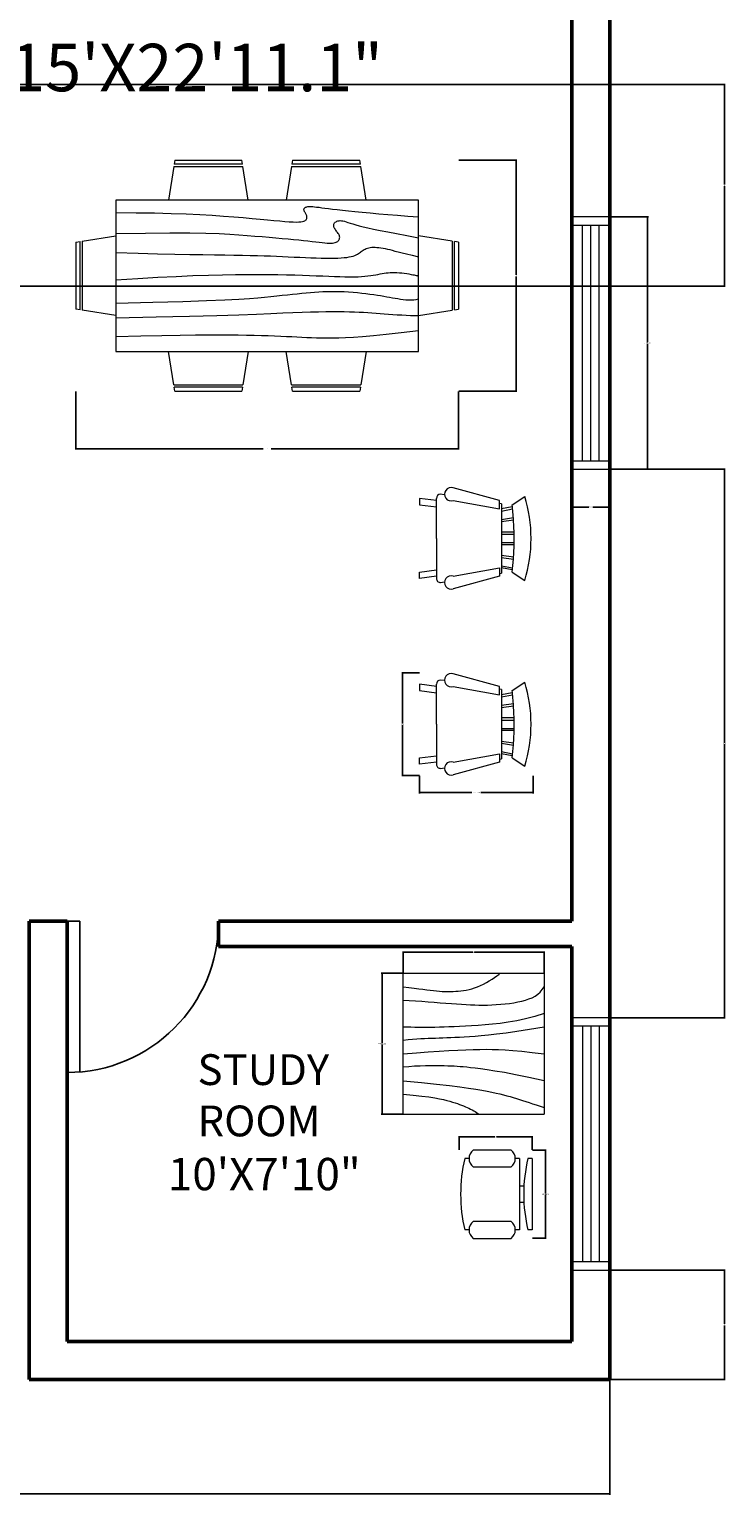
# Model space of a CAD drawing. Units: inches. Extents: x 16 to 443, y 39 to 637.
# Tile 2 of 3: x 278 to 443, y 39 to 387. Entities that reach past the tile are written whole.
import ezdxf

# ---------------------------------------------------------------- set-up
doc = ezdxf.new("R2010")
doc.units = ezdxf.units.IN
for name, color, linetype, lineweight in [('A-ANNO-DIMS', 2, 'Continuous', 18), ('A-AREA-IDEN', 7, 'Continuous', 18), ('A-DOOR', 3, 'Continuous', 25), ('A-FURN', 8, 'Continuous', 18), ('A-GLAZ', 4, 'Continuous', 18), ('A-WALL', 7, 'Continuous', 50)]:
    doc.layers.add(name, color=color, linetype=linetype, lineweight=lineweight)
doc.styles.get("Standard").update_dxf_attribs({"font": 'arial.ttf'})
doc.dimstyles.get("Standard").update_dxf_attribs({"dimtxt": 0.18, "dimasz": 0.18, "dimexe": 0.18, "dimexo": 0.0625, "dimgap": 0.09, "dimtad": 0, "dimtih": 1, "dimtoh": 1, "dimdec": 4, "dimzin": 0, "dimdsep": 46, "dimtxsty": 'Standard', "dimcen": 0.09, "dimadec": 0, "dimazin": 0, "dimtfac": 1, "dimtdec": 4, "dimtofl": 0, "dimtmove": 0, "dimatfit": 3, "dimfxl": 1, "dimtolj": 1, "dimtzin": 0, "dimarcsym": 0})

# ---------------------------------------------------------------- blocks, each defined once
blk = doc.blocks.new('Dining Set - 36 x 72 in.')
for p, q in [((-22.2343, 26.00059), (-23.4847, 17.99762)), ((-22.2304, 26), (-5.7608, 26)), ((-22, 27.5), (-22.1562, 26.50042)), ((-5.8416, 26.5), (-22.1534, 26.5)), ((-22, 27.5), (-6, 27.5)), ((-5.8437, 26.49966), (-6, 27.5)), ((-4.5152, 17.99762), (-5.7655, 25.99926)), ((5.7657, 26.00059), (4.5153, 17.99762)), ((5.7696, 26), (22.2392, 26)), ((6, 27.5), (5.8438, 26.50042)), ((22.1584, 26.5), (5.8466, 26.5)), ((6, 27.5), (22, 27.5)), ((22.1563, 26.49966), (22, 27.5)), ((23.4848, 17.99762), (22.2345, 25.99926)), ((36, 18), (-36, 18)), ((-36, 18), (-36, -18)), ((36, -18), (36, 18)), ((-45.5, 8), (-44.5004, 8.15617)), ((-45.5, 8), (-45.5, -8)), ((-44.5, -8.15843), (-44.5, 8.15338)), ((-44.0006, 8.23428), (-35.9976, 9.48474)), ((-44, 8.23041), (-44, -8.23915)), ((44.0006, 8.23428), (35.9976, 9.48474)), ((44, 8.23041), (44, -8.23915)), ((44.5, -8.15843), (44.5, 8.15338)), ((45.5, 8), (44.5005, 8.15617)), ((45.5, 8), (45.5, -8)), ((-44.4997, -8.15631), (-45.5, -8)), ((-35.9976, -9.48476), (-43.9993, -8.2345)), ((35.9976, -9.48476), (43.9993, -8.2345)), ((44.4997, -8.15631), (45.5, -8)), ((-36, -18), (36, -18)), ((-22.2343, -26.0006), (-23.4847, -17.99762)), ((-4.5152, -17.99762), (-5.7655, -25.99928)), ((5.7657, -26.0006), (4.5153, -17.99762)), ((23.4848, -17.99762), (22.2345, -25.99928)), ((-22.2304, -26), (-5.7608, -26)), ((-22, -27.5), (-22.1562, -26.50044)), ((-5.8416, -26.5), (-22.1534, -26.5)), ((-22, -27.5), (-6, -27.5)), ((-5.8437, -26.49967), (-6, -27.5)), ((5.7696, -26), (22.2392, -26)), ((6, -27.5), (5.8438, -26.50044)), ((22.1584, -26.5), (5.8466, -26.5)), ((6, -27.5), (22, -27.5)), ((22.1563, -26.49967), (22, -27.5))]:
    blk.add_line(p, q)
for points in [[(-36, 15), (-31.1772, 14.97754), (-26.8079, 14.91406), (-22.8538, 14.81543), (-19.276, 14.6875), (-16.0362, 14.53613), (-13.0957, 14.36718), (-10.4159, 14.18652), (-7.9583, 14), (-5.6904, 13.81315), (-3.6035, 13.63021), (-1.6954, 13.45508), (0.0365, 13.29166), (1.5945, 13.14388), (2.9811, 13.01562), (4.1988, 12.9108), (5.25, 12.83333), (6.1393, 12.78613), (6.8802, 12.76823), (7.4883, 12.77767), (7.9792, 12.8125), (8.3685, 12.87077), (8.6719, 12.95052), (8.9049, 13.0498), (9.0833, 13.16666), (9.2205, 13.29899), (9.3216, 13.44401), (9.3895, 13.59879), (9.4271, 13.76041), (9.4373, 13.92594), (9.4232, 14.09245), (9.3875, 14.257), (9.3333, 14.41666), (9.2638, 14.56917), (9.1836, 14.71484), (9.0975, 14.85465), (9.0104, 14.98958), (8.9272, 15.1206), (8.8529, 15.2487), (8.7922, 15.37483), (8.75, 15.5), (8.7305, 15.62467), (8.7344, 15.74739), (8.7617, 15.86621), (8.8125, 15.97916), (8.8867, 16.08431), (8.9844, 16.17968), (9.1055, 16.26334), (9.25, 16.33333), (9.4189, 16.38802), (9.6172, 16.42708), (9.8506, 16.45052), (10.125, 16.45833), (10.4463, 16.45052), (10.8203, 16.42708), (11.2529, 16.38802), (11.75, 16.33333), (12.3184, 16.26318), (12.9694, 16.17838), (13.7151, 16.07991), (14.5677, 15.96875), (15.5395, 15.84586), (16.6426, 15.71224), (17.8893, 15.56884), (19.2917, 15.41666), (20.859, 15.25667), (22.5879, 15.08984), (24.4721, 14.91715), (26.5052, 14.73958), (28.6809, 14.5581), (30.9929, 14.3737), (33.4347, 14.18733), (36, 14)], [(-36, 10), (-28.9766, 10.14274), (-23.1725, 10.20442), (-18.4241, 10.19775), (-14.5677, 10.13541), (-11.4399, 10.03011), (-8.877, 9.89453), (-6.7154, 9.74137), (-4.7917, 9.58333), (-2.9698, 9.43082), (-1.2246, 9.28515), (0.4415, 9.14534), (2.026, 9.01041), (3.5266, 8.87939), (4.9408, 8.7513), (6.266, 8.62516), (7.5, 8.5), (8.6411, 8.37549), (9.6914, 8.2539), (10.6538, 8.13818), (11.5312, 8.03125), (12.3267, 7.93603), (13.043, 7.85547), (13.6831, 7.79248), (14.25, 7.75), (14.7471, 7.7303), (15.1797, 7.73307), (15.5537, 7.75732), (15.875, 7.80208), (16.1494, 7.86637), (16.3828, 7.94922), (16.5811, 8.04964), (16.75, 8.16666), (16.8944, 8.29915), (17.0143, 8.44531), (17.1089, 8.60319), (17.1771, 8.77083), (17.218, 8.94629), (17.2305, 9.1276), (17.2137, 9.31282), (17.1667, 9.5), (17.0895, 9.6875), (16.987, 9.875), (16.8649, 10.0625), (16.7292, 10.25), (16.5856, 10.4375), (16.4401, 10.625), (16.2985, 10.8125), (16.1667, 11), (16.05, 11.18733), (15.9518, 11.3737), (15.8752, 11.5581), (15.8229, 11.73958), (15.798, 11.91715), (15.8034, 12.08984), (15.842, 12.25667), (15.9167, 12.41666), (16.0295, 12.56836), (16.1784, 12.70833), (16.3605, 12.83268), (16.5729, 12.9375), (16.8127, 13.01888), (17.0768, 13.07291), (17.3625, 13.0957), (17.6667, 13.08333), (17.9894, 13.03312), (18.3418, 12.94726), (18.7382, 12.82918), (19.1927, 12.68229), (19.7195, 12.51001), (20.3327, 12.31575), (21.0465, 12.10294), (21.875, 11.875), (22.8357, 11.63354), (23.959, 11.37304), (25.2786, 11.08618), (26.8282, 10.76562), (28.6414, 10.40405), (30.752, 9.99414), (33.1936, 9.52856), (36, 9)], [(-36, 5.5), (-30.7157, 5.3348), (-26.069, 5.20963), (-21.9946, 5.11767), (-18.4271, 5.05208), (-15.3009, 5.00602), (-12.5508, 4.97265), (-10.1112, 4.94515), (-7.9167, 4.91666), (-5.909, 4.88167), (-4.0586, 4.83984), (-2.3429, 4.79215), (-0.7396, 4.73958), (0.7739, 4.6831), (2.22, 4.6237), (3.6213, 4.56233), (5, 4.5), (6.373, 4.43782), (7.7344, 4.3776), (9.0723, 4.32129), (10.375, 4.27083), (11.6309, 4.22819), (12.8281, 4.19531), (13.9551, 4.17415), (15, 4.16666), (15.954, 4.17448), (16.819, 4.19791), (17.6001, 4.23698), (18.3021, 4.29166), (18.9299, 4.36198), (19.4883, 4.44791), (19.9823, 4.54948), (20.4167, 4.66666), (20.7969, 4.79899), (21.1302, 4.94401), (21.4245, 5.09879), (21.6875, 5.26041), (21.9271, 5.42594), (22.1511, 5.59245), (22.3672, 5.757), (22.5834, 5.91666), (22.8065, 6.06868), (23.0404, 6.21093), (23.2879, 6.34147), (23.5521, 6.45833), (23.8358, 6.55957), (24.142, 6.64323), (24.4735, 6.70735), (24.8334, 6.75), (25.2235, 6.76969), (25.642, 6.76692), (26.0858, 6.74267), (26.5521, 6.69791), (27.0379, 6.63362), (27.5404, 6.55078), (28.0565, 6.45036), (28.5834, 6.33333), (29.1242, 6.19987), (29.7071, 6.04687), (30.3661, 5.87044), (31.1354, 5.66666), (32.0493, 5.43164), (33.142, 5.16146), (34.4475, 4.85221), (36, 4.5)], [(-36, -1), (-30.7915, -0.6591), (-26.0195, -0.38216), (-21.6519, -0.16284), (-17.6563, 0.00521), (-14.0005, 0.12833), (-10.6523, 0.21289), (-7.5796, 0.26522), (-4.75, 0.29166), (-2.134, 0.29793), (0.2878, 0.28711), (2.5317, 0.26163), (4.6146, 0.22396), (6.5529, 0.17651), (8.3633, 0.12174), (10.0623, 0.06209), (11.6667, 0), (13.1899, -0.06201), (14.6341, -0.1211), (15.9982, -0.17432), (17.2813, -0.21875), (18.4823, -0.25147), (19.6003, -0.26953), (20.6343, -0.27002), (21.5834, -0.25), (22.4481, -0.20768), (23.2357, -0.14584), (23.9549, -0.06836), (24.6146, 0.02083), (25.2235, 0.11784), (25.7904, 0.21875), (26.3241, 0.31966), (26.8334, 0.41666), (27.3265, 0.50618), (27.8099, 0.58593), (28.2894, 0.65397), (28.7709, 0.70833), (29.2601, 0.74707), (29.763, 0.76823), (30.2855, 0.76985), (30.8334, 0.75), (31.4088, 0.70784), (31.9994, 0.64713), (32.589, 0.57275), (33.1615, 0.48958), (33.7008, 0.4025), (34.1908, 0.3164), (34.6153, 0.23616), (34.9584, 0.16666), (35.2099, 0.11165), (35.3848, 0.07031), (35.504, 0.04069), (35.5886, 0.02083), (35.6594, 0.00879), (35.7377, 0.0026), (35.8442, 0.00032), (36, 0)], [(-36, -6.5), (-27.1843, -6.31267), (-20.084, -6.1263), (-14.469, -5.9419), (-10.1094, -5.76042), (-6.7752, -5.58285), (-4.2363, -5.41016), (-2.2629, -5.24333), (-0.625, -5.08334), (0.8708, -4.93099), (2.2715, -4.78646), (3.5872, -4.64974), (4.8281, -4.52084), (6.0046, -4.39974), (7.127, -4.28646), (8.2053, -4.18099), (9.25, -4.08334), (10.2705, -3.99382), (11.2734, -3.91407), (12.2647, -3.84603), (13.25, -3.79167), (14.2354, -3.75293), (15.2266, -3.73177), (16.2295, -3.73015), (17.25, -3.75), (18.2912, -3.79248), (19.3451, -3.85547), (20.4009, -3.93604), (21.4479, -4.03125), (22.4754, -4.13819), (23.4727, -4.25391), (24.4289, -4.37549), (25.3334, -4.5), (26.1785, -4.62492), (26.9694, -4.74935), (27.7145, -4.87281), (28.4219, -4.99479), (29.1, -5.11483), (29.7572, -5.23242), (30.4016, -5.34709), (31.0417, -5.45834), (31.6837, -5.56437), (32.3262, -5.65821), (32.9658, -5.73153), (33.599, -5.77604), (34.2224, -5.78345), (34.8327, -5.74545), (35.4264, -5.65373), (36, -5.5)], [(-36, -10), (-26.4022, -9.81299), (-18.4675, -9.62891), (-11.9839, -9.45069), (-6.7396, -9.28125), (-2.5226, -9.12354), (0.8789, -8.98047), (3.6769, -8.85498), (6.0833, -8.75), (8.2767, -8.66765), (10.3021, -8.60677), (12.1712, -8.56543), (13.8958, -8.54167), (15.4876, -8.53353), (16.9583, -8.53907), (18.3197, -8.55632), (19.5834, -8.58334), (20.7616, -8.61841), (21.8685, -8.66081), (22.9188, -8.71004), (23.9271, -8.76563), (24.9081, -8.82707), (25.8763, -8.89388), (26.8465, -8.96558), (27.8334, -9.04167), (28.8474, -9.12118), (29.8828, -9.20117), (30.93, -9.27824), (31.9792, -9.34896), (33.0205, -9.40991), (34.0443, -9.45768), (35.0407, -9.48885), (36, -9.5)], [(-36, -14.5), (-30.0881, -14.33513), (-25.0332, -14.21224), (-20.7312, -14.12647), (-17.0781, -14.07292), (-13.97, -14.04671), (-11.3027, -14.04297), (-8.9724, -14.05681), (-6.875, -14.08334), (-4.9224, -14.11833), (-3.0905, -14.16016), (-1.3709, -14.20785), (0.2448, -14.26042), (1.7647, -14.3169), (3.1973, -14.3763), (4.5507, -14.43767), (5.8333, -14.5), (7.0554, -14.5621), (8.235, -14.62175), (9.3922, -14.67652), (10.5469, -14.72396), (11.7192, -14.76164), (12.929, -14.78711), (14.1965, -14.79794), (15.5417, -14.79167), (16.9933, -14.76424), (18.6152, -14.70508), (20.4804, -14.60197), (22.6615, -14.44271), (25.2312, -14.21509), (28.2624, -13.9069), (31.8277, -13.50594), (36, -13)]]:
    blk.add_lwpolyline(points)
blk = doc.blocks.new('Chair - Rocking')
for p, q in [((-8, -4.5), (-10, -1.5)), ((8, -4.5), (10, -1.5)), ((-7.5, -4.5), (-7, -7)), ((-6.5, -7), (-7.02225, -4.43)), ((-4.5, -7), (-4.96674, -4.19951)), ((-4, -7), (-4.40532, -4.16272)), ((-1.5, -4.05012), (-1.5, -7)), ((-1, -7), (-1, -4.05012)), ((1, -7), (1, -4.04655)), ((1.5, -4.05012), (1.5, -7)), ((4, -7), (4.40187, -4.18694)), ((4.5, -7), (4.96761, -4.19437)), ((6.5, -7), (7, -4.4057)), ((7.5, -4.5), (7, -7)), ((-9, -7.5), (-12, -18.49999)), ((-7, -7.5), (-9, -7.5)), ((-9, -18.49999), (-7, -7.5)), ((-8.23428, -6.99939), (-8.3093, -7.47958)), ((-8.23041, -7), (8.23915, -7)), ((7, -7.5), (9, -7.5)), ((9, -18.49999), (7, -7.5)), ((8.31071, -7.48854), (8.23449, -7.00073)), ((9, -7.5), (12, -18.49999)), ((-10.36644, -20.64523), (-10.5, -21.49999)), ((10.5, -21.49999), (10.3575, -20.58798)), ((-9, -22.49999), (-9.5, -26.49999)), ((0, -22.49999), (-9.5, -22.49999)), ((-8, -26.49999), (-7.5, -22.49999)), ((0, -22.49999), (9.5, -22.49999)), ((8, -26.49999), (7.5, -22.49999)), ((9, -22.49999), (9.5, -26.49999)), ((-9.5, -26.49999), (-8, -26.49999)), ((9.5, -26.49999), (8, -26.49999))]:
    blk.add_line(p, q)
for centre, radius, start, end in [((0, -34.08333), 34.08333, 72.93847, 107.0615), ((0, -68.25004), 64.25, 93.92211, 97.15267), ((0, -68.25004), 64.25, 82.84733, 93.92211), ((-10.5, -18.99999), 1.58114, 161.5651, 18.43495), ((10.5, -18.99999), 1.58114, 161.5651, 18.43495), ((-9.5, -21.49999), 1, 180, 270), ((9.5, -21.49999), 1, 270, 0)]:
    blk.add_arc(centre, radius, start, end)
blk = doc.blocks.new('Chair - Desk')
for p, q in [((-8.5, 0), (-8.5, -1)), ((-8.5, 0), (8.5, 0)), ((8.5, 0), (8.5, -1)), ((-8.5, -3), (-8.5, -4)), ((-8.5, -3), (8.5, -3)), ((-2, -3), (-2, -1.9355)), ((2, -1.9576), (2, -3)), ((8.5, -3), (8.5, -4)), ((-10.5, -5), (-10.5, -14)), ((-6.5, -14), (-6.5, -5)), ((6.5, -5), (6.5, -14)), ((10.5, -14), (10.5, -5)), ((-8.5, -15), (-8.5, -16)), ((8.5, -15), (8.5, -16))]:
    blk.add_line(p, q)
for centre, radius, start, end in [((0, 34.625), 36.625, 256.5803, 283.4197), ((-8.5, -6.5), 2.5, 36.8699, 143.1301), ((8.5, -6.5), 2.5, 36.8699, 143.1301), ((-8.5, -12.5), 2.5, 216.8699, 323.1301), ((0, 19.625), 36.625, 256.5803, 283.4197), ((8.5, -12.5), 2.5, 216.8699, 323.1301)]:
    blk.add_arc(centre, radius, start, end)
blk = doc.blocks.new('Table - Square Woodgrain 42 x 42 in.')
blk.add_line((0, -42), (42, -42))
for points in [[(0, -4), (1.704, -4.2172), (3.2358, -4.4188), (4.615, -4.604), (5.8615, -4.7721), (6.9951, -4.9224), (8.0357, -5.0541), (9.0031, -5.1667), (9.9171, -5.2594), (10.7951, -5.3316), (11.6445, -5.3836), (12.4702, -5.4157), (13.277, -5.4283), (14.0698, -5.4217), (14.8535, -5.3964), (15.6331, -5.3526), (16.4133, -5.2908), (17.1986, -5.2103), (17.9913, -5.1062), (18.793, -4.9727), (19.6056, -4.8038), (20.4307, -4.5937), (21.2701, -4.3365), (22.1256, -4.0262), (22.9989, -3.6571), (23.888, -3.2272), (24.7756, -2.7516), (25.6408, -2.2491), (26.4624, -1.7387), (27.2195, -1.2395), (27.891, -0.7703), (28.456, -0.3501), (28.8934, 0.002)], [(0, -42), (0, 0), (42, 0), (42, -42)], [(0, -8), (1.8203, -8.1001), (3.6741, -8.2149), (5.5411, -8.3408), (7.4011, -8.4741), (9.2339, -8.6112), (11.0193, -8.7484), (12.7371, -8.8821), (14.3671, -9.0086), (15.8954, -9.1246), (17.3337, -9.2278), (18.6997, -9.3159), (20.0116, -9.387), (21.2871, -9.4389), (22.5442, -9.4696), (23.8008, -9.477), (25.0749, -9.459), (26.3791, -9.4137), (27.7049, -9.3403), (29.0383, -9.2382), (30.3655, -9.1068), (31.6728, -8.9455), (32.9461, -8.7535), (34.1717, -8.5304), (35.3358, -8.2756), (36.4268, -7.9863), (37.443, -7.6521), (38.3849, -7.2603), (39.253, -6.7986), (40.048, -6.2542), (40.7705, -5.6147), (41.421, -4.8674), (42, -4)], [(42, -12), (39.1784, -12.8621), (36.4519, -13.5654), (33.8246, -14.1294), (31.3004, -14.5731), (28.8832, -14.9161), (26.577, -15.1775), (24.3858, -15.3768), (22.3136, -15.5332), (20.3622, -15.6632), (18.5254, -15.7718), (16.7947, -15.8612), (15.1618, -15.9338), (13.6183, -15.9916), (12.1558, -16.0369), (10.7659, -16.0718), (9.4403, -16.0987), (8.1703, -16.1191), (6.9461, -16.1325), (5.7577, -16.1377), (4.595, -16.1335), (3.4479, -16.1188), (2.3064, -16.0924), (1.1604, -16.0532), (0, -16)], [(42, -16), (37.6529, -16.7365), (33.8802, -17.329), (30.6179, -17.7961), (27.8015, -18.1561), (25.3668, -18.4275), (23.2497, -18.6288), (21.3859, -18.7785), (19.7111, -18.8949), (18.1693, -18.9939), (16.7375, -19.0795), (15.401, -19.1534), (14.1449, -19.217), (12.9544, -19.2717), (11.8148, -19.3191), (10.7113, -19.3606), (9.6291, -19.3976), (8.5534, -19.4323), (7.47, -19.4689), (6.3643, -19.5122), (5.222, -19.5672), (4.0288, -19.6386), (2.7703, -19.7313), (1.4321, -19.8501), (0, -20)], [(0, -24), (3.9243, -23.6805), (7.4766, -23.4138), (10.6891, -23.1954), (13.5943, -23.0205), (16.2247, -22.8847), (18.6125, -22.7832), (20.7903, -22.7116), (22.7903, -22.6651), (24.6563, -22.642), (26.4764, -22.6507), (28.35, -22.7024), (30.3766, -22.8084), (32.6555, -22.98), (35.2861, -23.2283), (38.3678, -23.5645), (42, -24)], [(42, -32), (37.392, -31.017), (33.4585, -30.2231), (30.1291, -29.5949), (27.3334, -29.109), (25.0009, -28.742), (23.0612, -28.4707), (21.4439, -28.2716), (20.0786, -28.1215), (18.8998, -28.0002), (17.8609, -27.9014), (16.9206, -27.8219), (16.0371, -27.7588), (15.1691, -27.709), (14.2748, -27.6693), (13.3128, -27.6368), (12.2415, -27.6083), (11.0295, -27.5824), (9.6867, -27.5643), (8.233, -27.5608), (6.6884, -27.5787), (5.0728, -27.6248), (3.4062, -27.7058), (1.7086, -27.8286), (0, -28)], [(0, -32), (5.4026, -32.5358), (9.9494, -33.019), (13.7424, -33.4553), (16.8834, -33.8505), (19.4743, -34.2106), (21.6171, -34.5413), (23.4136, -34.8486), (24.9657, -35.1382), (26.3614, -35.4156), (27.6332, -35.6841), (28.7995, -35.9467), (29.8788, -36.2064), (30.8897, -36.4661), (31.8507, -36.7288), (32.7802, -36.9973), (33.6968, -37.2747), (34.6175, -37.5635), (35.5531, -37.8651), (36.5128, -38.1805), (37.506, -38.5108), (38.5421, -38.8568), (39.6302, -39.2197), (40.7797, -39.6004), (42, -40)], [(0, -36), (3.0098, -36.2857), (5.5354, -36.5643), (7.6368, -36.8359), (9.374, -37.1009), (10.807, -37.3597), (11.9957, -37.6126), (13.0002, -37.8599), (13.8804, -38.102), (14.6874, -38.3393), (15.4365, -38.5729), (16.1338, -38.8041), (16.7858, -39.0341), (17.3987, -39.264), (17.9787, -39.4952), (18.5322, -39.7288), (19.0655, -39.9662), (19.5832, -40.2081), (20.0842, -40.4544), (20.5657, -40.7046), (21.0249, -40.9581), (21.459, -41.2144), (21.8653, -41.4731), (22.2409, -41.7335), (22.5831, -41.9951)]]:
    blk.add_lwpolyline(points)
blk = doc.blocks.new('WIN-60IN')
for p, q in [((0, 60), (0, 0)), ((9, 60), (0, 60)), ((9, 0), (9, 60)), ((9, 58), (0, 58)), ((2.5, 58), (2.5, 2)), ((4.5, 58), (4.5, 2)), ((6.5, 58), (6.5, 2)), ((0, 2), (9, 2)), ((0, 0), (9, 0))]:
    blk.add_line(p, q)
blk = doc.blocks.new('DOOR-SINGLE-36IN')
for p, q in [((33, 36), (33, 0)), ((36, 36), (36, 0)), ((36, 0), (33, 0))]:
    blk.add_line(p, q)
blk.add_arc((36, 0), 36, 90, 180)
blk = doc.blocks.new('*D15')
at = {"layer": 'A-ANNO-DIMS', "color": 0, "lineweight": -2, "transparency": 16777216}
for p, q in [((415.81, 342.58), (424.93, 342.58)), ((424.75, 342.4), (424.75, 312.76)), ((424.75, 282.76), (424.75, 312.4)), ((415.81, 282.58), (424.93, 282.58))]:
    blk.add_line(p, q, dxfattribs=at)
at = {"layer": 'A-ANNO-DIMS', "color": 0, "transparency": 16777216}
for points in [[(424.72, 342.4), (424.78, 342.4), (424.75, 342.58)], [(424.72, 282.76), (424.78, 282.76), (424.75, 282.58)]]:
    blk.add_solid(points, dxfattribs=at)
at = {"layer": 'Defpoints', "color": 0, "transparency": 16777216}
for p in [(415.75, 342.58), (415.75, 282.58), (424.75, 282.58)]:
    blk.add_point(p, dxfattribs=at)
at = {"layer": 'A-ANNO-DIMS', "color": 0, "transparency": 16777216, "insert": (424.75, 312.58), "char_height": 0.18, "attachment_point": 5}
blk.add_mtext('\\A1;WINDOW 60 TYP.', dxfattribs=at)
blk = doc.blocks.new('*D16')
at = {"layer": 'A-ANNO-DIMS', "color": 0, "lineweight": -2, "transparency": 16777216}
for p, q in [((406.75, 282.52), (406.75, 273.4)), ((415.75, 282.52), (415.75, 273.4)), ((406.93, 273.58), (410.79, 273.58)), ((415.57, 273.58), (411.71, 273.58))]:
    blk.add_line(p, q, dxfattribs=at)
at = {"layer": 'A-ANNO-DIMS', "color": 0, "transparency": 16777216}
for points in [[(406.93, 273.61), (406.93, 273.55), (406.75, 273.58)], [(415.57, 273.61), (415.57, 273.55), (415.75, 273.58)]]:
    blk.add_solid(points, dxfattribs=at)
at = {"layer": 'Defpoints', "color": 0, "transparency": 16777216}
for p in [(406.75, 282.58), (415.75, 282.58), (406.75, 273.58)]:
    blk.add_point(p, dxfattribs=at)
at = {"layer": 'A-ANNO-DIMS', "color": 0, "transparency": 16777216, "insert": (411.25, 273.58), "char_height": 0.18, "attachment_point": 5}
blk.add_mtext('\\A1;9 TYP.', dxfattribs=at)
blk = doc.blocks.new('*D29')
at = {"layer": 'A-ANNO-DIMS', "color": 0, "lineweight": -2, "transparency": 16777216}
for p, q in [((370.54, 209.63), (370.54, 205.47)), ((397.54, 209.63), (397.54, 205.47)), ((370.72, 205.65), (382.94, 205.65)), ((397.36, 205.65), (385.13, 205.65))]:
    blk.add_line(p, q, dxfattribs=at)
at = {"layer": 'A-ANNO-DIMS', "color": 0, "transparency": 16777216}
for points in [[(370.72, 205.68), (370.72, 205.62), (370.54, 205.65)], [(397.36, 205.68), (397.36, 205.62), (397.54, 205.65)]]:
    blk.add_solid(points, dxfattribs=at)
at = {"layer": 'Defpoints', "color": 0, "transparency": 16777216}
for p in [(370.54, 209.7), (397.54, 209.7), (397.54, 205.65)]:
    blk.add_point(p, dxfattribs=at)
at = {"layer": 'A-ANNO-DIMS', "color": 0, "transparency": 16777216, "insert": (384.04, 205.65), "char_height": 0.18, "attachment_point": 5}
blk.add_mtext('\\A1;ROCKER 27 TYP.', dxfattribs=at)
blk = doc.blocks.new('*D30')
at = {"layer": 'A-ANNO-DIMS', "color": 0, "lineweight": -2, "transparency": 16777216}
for p, q in [((370.48, 234.13), (366.31, 234.13)), ((366.49, 233.95), (366.49, 222.09)), ((366.49, 209.88), (366.49, 221.73)), ((370.48, 209.7), (366.31, 209.7))]:
    blk.add_line(p, q, dxfattribs=at)
at = {"layer": 'A-ANNO-DIMS', "color": 0, "transparency": 16777216}
for points in [[(366.46, 233.95), (366.52, 233.95), (366.49, 234.13)], [(366.46, 209.88), (366.52, 209.88), (366.49, 209.7)]]:
    blk.add_solid(points, dxfattribs=at)
at = {"layer": 'Defpoints', "color": 0, "transparency": 16777216}
for p in [(370.54, 234.13), (366.49, 209.7), (370.54, 209.7)]:
    blk.add_point(p, dxfattribs=at)
at = {"layer": 'A-ANNO-DIMS', "color": 0, "transparency": 16777216, "insert": (366.49, 221.91), "char_height": 0.18, "attachment_point": 5}
blk.add_mtext('\\A1;24 TYP.', dxfattribs=at)
blk = doc.blocks.new('*D33')
at = {"layer": 'A-ANNO-DIMS', "color": 0, "lineweight": -2, "transparency": 16777216}
for p, q in [((288.81, 301.05), (288.81, 287.28)), ((379.81, 301.05), (379.81, 287.28)), ((288.99, 287.46), (333.36, 287.46)), ((379.63, 287.46), (335.26, 287.46))]:
    blk.add_line(p, q, dxfattribs=at)
at = {"layer": 'A-ANNO-DIMS', "color": 0, "transparency": 16777216}
for points in [[(288.99, 287.49), (288.99, 287.43), (288.81, 287.46)], [(379.63, 287.49), (379.63, 287.43), (379.81, 287.46)]]:
    blk.add_solid(points, dxfattribs=at)
at = {"layer": 'Defpoints', "color": 0, "transparency": 16777216}
for p in [(288.81, 301.11), (379.81, 301.11), (379.81, 287.46)]:
    blk.add_point(p, dxfattribs=at)
at = {"layer": 'A-ANNO-DIMS', "color": 0, "transparency": 16777216, "insert": (334.31, 287.46), "char_height": 0.18, "attachment_point": 5}
blk.add_mtext('\\A1;DINING SET 91', dxfattribs=at)
blk = doc.blocks.new('*D34')
at = {"layer": 'A-ANNO-DIMS', "color": 0, "lineweight": -2, "transparency": 16777216}
for p, q in [((379.87, 356.11), (393.64, 356.11)), ((393.46, 355.93), (393.46, 328.79)), ((393.46, 301.29), (393.46, 328.43)), ((379.87, 301.11), (393.64, 301.11))]:
    blk.add_line(p, q, dxfattribs=at)
at = {"layer": 'A-ANNO-DIMS', "color": 0, "transparency": 16777216}
for points in [[(393.43, 355.93), (393.49, 355.93), (393.46, 356.11)], [(393.43, 301.29), (393.49, 301.29), (393.46, 301.11)]]:
    blk.add_solid(points, dxfattribs=at)
at = {"layer": 'Defpoints', "color": 0, "transparency": 16777216}
for p in [(379.81, 356.11), (393.46, 356.11), (379.81, 301.11)]:
    blk.add_point(p, dxfattribs=at)
at = {"layer": 'A-ANNO-DIMS', "color": 0, "transparency": 16777216, "insert": (393.46, 328.61), "char_height": 0.18, "attachment_point": 5}
blk.add_mtext('\\A1;55', dxfattribs=at)
blk = doc.blocks.new('*D41')
at = {"layer": 'A-ANNO-DIMS', "color": 0, "lineweight": -2, "transparency": 16777216}
for p, q in [((397.35, 120.63), (400.62, 120.63)), ((400.44, 120.45), (400.44, 110.31)), ((400.44, 99.81), (400.44, 109.94)), ((397.35, 99.63), (400.62, 99.63))]:
    blk.add_line(p, q, dxfattribs=at)
at = {"layer": 'A-ANNO-DIMS', "color": 0, "transparency": 16777216}
for points in [[(400.41, 120.45), (400.47, 120.45), (400.44, 120.63)], [(400.41, 99.81), (400.47, 99.81), (400.44, 99.63)]]:
    blk.add_solid(points, dxfattribs=at)
at = {"layer": 'Defpoints', "color": 0, "transparency": 16777216}
for p in [(397.29, 120.63), (397.29, 99.63), (400.44, 99.63)]:
    blk.add_point(p, dxfattribs=at)
at = {"layer": 'A-ANNO-DIMS', "color": 0, "transparency": 16777216, "insert": (400.44, 110.13), "char_height": 0.18, "attachment_point": 5}
blk.add_mtext('\\A1;DESK CHAIR 21', dxfattribs=at)
blk = doc.blocks.new('*D42')
at = {"layer": 'A-ANNO-DIMS', "color": 0, "lineweight": -2, "transparency": 16777216}
for p, q in [((379.95, 120.69), (379.95, 123.96)), ((380.13, 123.78), (388.41, 123.78)), ((397.11, 123.78), (388.83, 123.78)), ((397.29, 120.69), (397.29, 123.96))]:
    blk.add_line(p, q, dxfattribs=at)
at = {"layer": 'A-ANNO-DIMS', "color": 0, "transparency": 16777216}
for points in [[(380.13, 123.81), (380.13, 123.75), (379.95, 123.78)], [(397.11, 123.81), (397.11, 123.75), (397.29, 123.78)]]:
    blk.add_solid(points, dxfattribs=at)
at = {"layer": 'Defpoints', "color": 0, "transparency": 16777216}
for p in [(397.29, 123.78), (379.95, 120.63), (397.29, 120.63)]:
    blk.add_point(p, dxfattribs=at)
at = {"layer": 'A-ANNO-DIMS', "color": 0, "transparency": 16777216, "insert": (388.62, 123.78), "char_height": 0.18, "attachment_point": 5}
blk.add_mtext('\\A1;17', dxfattribs=at)
blk = doc.blocks.new('*D43')
at = {"layer": 'A-ANNO-DIMS', "color": 0, "lineweight": -2, "transparency": 16777216}
for p, q in [((366.58, 162.67), (361.43, 162.67)), ((361.61, 162.49), (361.61, 146.09)), ((361.61, 129.31), (361.61, 145.72)), ((366.58, 129.13), (361.43, 129.13))]:
    blk.add_line(p, q, dxfattribs=at)
at = {"layer": 'A-ANNO-DIMS', "color": 0, "transparency": 16777216}
for points in [[(361.58, 162.49), (361.64, 162.49), (361.61, 162.67)], [(361.58, 129.31), (361.64, 129.31), (361.61, 129.13)]]:
    blk.add_solid(points, dxfattribs=at)
at = {"layer": 'Defpoints', "color": 0, "transparency": 16777216}
for p in [(361.61, 162.67), (366.64, 162.67), (366.64, 129.13)]:
    blk.add_point(p, dxfattribs=at)
at = {"layer": 'A-ANNO-DIMS', "color": 0, "transparency": 16777216, "insert": (361.61, 145.9), "char_height": 0.18, "attachment_point": 5}
blk.add_mtext('\\A1;STUDY TABLE 34', dxfattribs=at)
blk = doc.blocks.new('*D44')
at = {"layer": 'A-ANNO-DIMS', "color": 0, "lineweight": -2, "transparency": 16777216}
for p, q in [((366.64, 162.73), (366.64, 167.88)), ((366.82, 167.7), (383.19, 167.7)), ((399.99, 167.7), (383.62, 167.7)), ((400.17, 162.73), (400.17, 167.88))]:
    blk.add_line(p, q, dxfattribs=at)
at = {"layer": 'A-ANNO-DIMS', "color": 0, "transparency": 16777216}
for points in [[(366.82, 167.73), (366.82, 167.67), (366.64, 167.7)], [(399.99, 167.73), (399.99, 167.67), (400.17, 167.7)]]:
    blk.add_solid(points, dxfattribs=at)
at = {"layer": 'Defpoints', "color": 0, "transparency": 16777216}
for p in [(400.17, 167.7), (366.64, 162.67), (400.17, 162.67)]:
    blk.add_point(p, dxfattribs=at)
at = {"layer": 'A-ANNO-DIMS', "color": 0, "transparency": 16777216, "insert": (383.41, 167.7), "char_height": 0.18, "attachment_point": 5}
blk.add_mtext('\\A1;34', dxfattribs=at)
blk = doc.blocks.new('*D45')
at = {"layer": 'A-ANNO-DIMS', "color": 0, "lineweight": -2, "transparency": 16777216}
for p, q in [((43.75, 165.02), (43.75, 38.65)), ((415.75, 66.02), (415.75, 38.65)), ((43.93, 38.83), (229.46, 38.83)), ((415.57, 38.83), (230.04, 38.83))]:
    blk.add_line(p, q, dxfattribs=at)
at = {"layer": 'A-ANNO-DIMS', "color": 0, "transparency": 16777216}
for points in [[(43.93, 38.86), (43.93, 38.8), (43.75, 38.83)], [(415.57, 38.86), (415.57, 38.8), (415.75, 38.83)]]:
    blk.add_solid(points, dxfattribs=at)
at = {"layer": 'Defpoints', "color": 0, "transparency": 16777216}
for p in [(43.75, 165.08), (415.75, 66.08), (415.75, 38.83)]:
    blk.add_point(p, dxfattribs=at)
at = {"layer": 'A-ANNO-DIMS', "color": 0, "transparency": 16777216, "insert": (229.75, 38.83), "char_height": 0.18, "attachment_point": 5}
blk.add_mtext('\\A1;372', dxfattribs=at)
blk = doc.blocks.new('*D56')
at = {"layer": 'A-ANNO-DIMS', "color": 0, "lineweight": -2, "transparency": 16777216}
for p, q in [((415.81, 92.08), (443.18, 92.08)), ((443, 91.9), (443, 79.26)), ((443, 66.26), (443, 78.9)), ((415.81, 66.08), (443.18, 66.08))]:
    blk.add_line(p, q, dxfattribs=at)
at = {"layer": 'A-ANNO-DIMS', "color": 0, "transparency": 16777216}
for points in [[(442.97, 91.9), (443.03, 91.9), (443, 92.08)], [(442.97, 66.26), (443.03, 66.26), (443, 66.08)]]:
    blk.add_solid(points, dxfattribs=at)
at = {"layer": 'Defpoints', "color": 0, "transparency": 16777216}
for p in [(415.75, 92.08), (443, 92.08), (415.75, 66.08)]:
    blk.add_point(p, dxfattribs=at)
at = {"layer": 'A-ANNO-DIMS', "color": 0, "transparency": 16777216, "insert": (443, 79.08), "char_height": 0.18, "attachment_point": 5}
blk.add_mtext('\\A1;26', dxfattribs=at)
blk = doc.blocks.new('*D57')
at = {"layer": 'A-ANNO-DIMS', "color": 0, "lineweight": -2, "transparency": 16777216}
for p, q in [((415.81, 282.58), (443.18, 282.58)), ((443, 282.4), (443, 217.51)), ((443, 152.26), (443, 217.15)), ((415.81, 152.08), (443.18, 152.08))]:
    blk.add_line(p, q, dxfattribs=at)
at = {"layer": 'A-ANNO-DIMS', "color": 0, "transparency": 16777216}
for points in [[(442.97, 282.4), (443.03, 282.4), (443, 282.58)], [(442.97, 152.26), (443.03, 152.26), (443, 152.08)]]:
    blk.add_solid(points, dxfattribs=at)
at = {"layer": 'Defpoints', "color": 0, "transparency": 16777216}
for p in [(415.75, 282.58), (443, 282.58), (415.75, 152.08)]:
    blk.add_point(p, dxfattribs=at)
at = {"layer": 'A-ANNO-DIMS', "color": 0, "transparency": 16777216, "insert": (443, 217.33), "char_height": 0.18, "attachment_point": 5}
blk.add_mtext('\\A1;130.5', dxfattribs=at)
blk = doc.blocks.new('*D62')
at = {"layer": 'A-ANNO-DIMS', "color": 0, "lineweight": -2, "transparency": 16777216}
for p, q in [((94.81, 374.08), (443.18, 374.08)), ((443, 373.9), (443, 350.26)), ((443, 326.26), (443, 349.9)), ((94.81, 326.08), (443.18, 326.08))]:
    blk.add_line(p, q, dxfattribs=at)
at = {"layer": 'A-ANNO-DIMS', "color": 0, "transparency": 16777216}
for points in [[(442.97, 373.9), (443.03, 373.9), (443, 374.08)], [(442.97, 326.26), (443.03, 326.26), (443, 326.08)]]:
    blk.add_solid(points, dxfattribs=at)
at = {"layer": 'Defpoints', "color": 0, "transparency": 16777216}
for p in [(94.75, 374.08), (443, 374.08), (94.75, 326.08)]:
    blk.add_point(p, dxfattribs=at)
at = {"layer": 'A-ANNO-DIMS', "color": 0, "transparency": 16777216, "insert": (443, 350.08), "char_height": 0.18, "attachment_point": 5}
blk.add_mtext('\\A1;48', dxfattribs=at)

msp = doc.modelspace()

# ---------------------------------------------------------------- linework, layer by layer
at = {"layer": 'A-WALL'}
for p, q in [((415.7492, 609.0801), (415.7492, 66.0801)), ((406.7492, 450.0801), (406.7492, 175.0801)), ((277.7492, 175.0801), (286.7492, 175.0801)), ((277.7492, 175.0801), (277.7492, 66.0801)), ((286.7492, 175.0801), (286.7492, 75.0801)), ((322.7492, 175.0801), (322.7492, 169.0801)), ((322.7492, 175.0801), (406.7492, 175.0801)), ((322.7492, 169.0801), (406.7492, 169.0801)), ((406.7492, 169.0801), (406.7492, 75.0801)), ((286.7492, 75.0801), (406.7492, 75.0801)), ((277.7492, 66.0801), (415.7492, 66.0801))]:
    msp.add_line(p, q, dxfattribs=at)

# ---------------------------------------------------------------- block references
at = {"layer": 'A-DOOR', "rotation": 180}
msp.add_blockref('DOOR-SINGLE-36IN', (322.7494, 175.0802), dxfattribs=at)
at = {"layer": 'A-FURN'}
msp.add_blockref('Dining Set - 36 x 72 in.', (334.3099, 328.6098), dxfattribs=at)
at = {"layer": 'A-FURN', "rotation": 270}
for name, p in [('Chair - Rocking', (397.0377, 266.1127)), ('Chair - Rocking', (397.0377, 221.9128)), ('Chair - Desk', (397.2873, 110.1273))]:
    msp.add_blockref(name, p, dxfattribs=at)
at = {"layer": 'A-FURN', "xscale": 0.7984530820493868, "yscale": 0.7984530820493868, "zscale": 0.7984530820493868}
msp.add_blockref('Table - Square Woodgrain 42 x 42 in.', (366.6384, 162.6691), dxfattribs=at)
at = {"layer": 'A-GLAZ', "rotation": 180}
msp.add_blockref('WIN-60IN', (415.7494, 342.5802), dxfattribs=at)
at = {"layer": 'A-GLAZ'}
msp.add_blockref('WIN-60IN', (406.749, 92.08), dxfattribs=at)

# ---------------------------------------------------------------- texts
at = {"layer": 'A-AREA-IDEN', "attachment_point": 1}
for s, width, gutter_width, insert, char_height in [('15\'X22\'11.1"', 769.796886, 56.4482, (273.0061, 383.7619), 11.289646), ('STUDY\\PROOM', 499.218487, 36.6071, (317.7395, 143.4187), 7.32141), ('10\'X7\'10"', 523.488138, 38.3867, (310.6861, 118.7548), 7.67734)]:
    msp.add_mtext_dynamic_manual_height_columns(s, width=width, gutter_width=gutter_width, heights=[0], dxfattribs=dict(at, insert=insert, char_height=char_height))

# ---------------------------------------------------------------- dimensions: what is measured, and where the dimension line sits
at = {"layer": 'A-ANNO-DIMS'}
for base, p1, p2, override, picture, middle in [((442.9992, 374.0801), (94.7492, 326.0801), (94.7492, 374.0801), {"dimdec": 0, "dimlfac": 1, "dimrnd": 0, "dimzin": 0, "dimdsep": 46, "dimlunit": 2}, '*D62', (442.9992, 350.0801)), ((393.4599, 356.1098), (379.8099, 301.1098), (379.8099, 356.1098), {"dimdec": 0, "dimlfac": 1, "dimrnd": 0, "dimzin": 0, "dimdsep": 46, "dimlunit": 2}, '*D34', (393.4599, 328.6098)), ((442.9992, 282.5801), (415.7492, 152.0801), (415.7492, 282.5801), {"dimdec": 1, "dimlfac": 1, "dimrnd": 0, "dimzin": 0, "dimdsep": 46, "dimlunit": 2}, '*D57', (442.9992, 217.3301)), ((442.9992, 92.0801), (415.7492, 66.0801), (415.7492, 92.0801), {"dimdec": 0, "dimlfac": 1, "dimrnd": 0, "dimzin": 0, "dimdsep": 46, "dimlunit": 2}, '*D56', (442.9992, 79.0801))]:
    dim = msp.add_linear_dim(base=base, p1=p1, p2=p2, angle=90, dimstyle='Standard', override=override, dxfattribs=at)
    dim.commit()
    dim.dimension.update_dxf_attribs({"geometry": picture, "text_midpoint": middle})
for base, p1, p2, angle, text, picture, middle in [((424.7492, 282.5801), (415.7492, 342.5801), (415.7492, 282.5801), 270, 'WINDOW <> TYP.', '*D15', (424.7492, 312.5801)), ((406.7492, 273.5801), (415.7492, 282.5801), (406.7492, 282.5801), 180, '<> TYP.', '*D16', (411.2492, 273.5801)), ((366.4877, 209.6953), (370.5377, 234.1303), (370.5377, 209.6953), 270, '<> TYP.', '*D30', (366.4877, 221.9128)), ((361.6079, 162.6707), (366.6384, 129.134), (366.6384, 162.6707), 90, 'STUDY TABLE <>', '*D43', (361.6079, 145.9024)), ((400.4373, 99.6273), (397.2873, 120.6273), (397.2873, 99.6273), 270, 'DESK CHAIR <>', '*D41', (400.4373, 110.1273))]:
    dim = msp.add_linear_dim(base=base, p1=p1, p2=p2, angle=angle, text=text, dimstyle='Standard', override={"dimdec": 0, "dimlfac": 1, "dimrnd": 0, "dimzin": 0, "dimdsep": 46, "dimlunit": 2}, dxfattribs=at)
    dim.commit()
    dim.dimension.update_dxf_attribs({"geometry": picture, "text_midpoint": middle})
for base, p1, p2, text, picture, middle in [((379.8099, 287.4598), (288.8099, 301.1098), (379.8099, 301.1098), 'DINING SET <>', '*D33', (334.3099, 287.4598)), ((397.5377, 205.6453), (370.5377, 209.6953), (397.5377, 209.6953), 'ROCKER <> TYP.', '*D29', (384.0377, 205.6453))]:
    dim = msp.add_linear_dim(base=base, p1=p1, p2=p2, text=text, dimstyle='Standard', override={"dimdec": 0, "dimlfac": 1, "dimrnd": 0, "dimzin": 0, "dimdsep": 46, "dimlunit": 2}, dxfattribs=at)
    dim.commit()
    dim.dimension.update_dxf_attribs({"geometry": picture, "text_midpoint": middle})
for base, p1, p2, picture, middle in [((400.1734, 167.7012), (366.6384, 162.6707), (400.1734, 162.6707), '*D44', (383.4059, 167.7012)), ((415.7492, 38.8301), (43.7492, 165.0801), (415.7492, 66.0801), '*D45', (229.7492, 38.8301)), ((397.2873, 123.7773), (379.954, 120.6273), (397.2873, 120.6273), '*D42', (388.6207, 123.7773))]:
    dim = msp.add_linear_dim(base=base, p1=p1, p2=p2, dimstyle='Standard', override={"dimdec": 0, "dimlfac": 1, "dimrnd": 0, "dimzin": 0, "dimdsep": 46, "dimlunit": 2}, dxfattribs=at)
    dim.commit()
    dim.dimension.update_dxf_attribs({"geometry": picture, "text_midpoint": middle})

doc.saveas('drawing.dxf')
